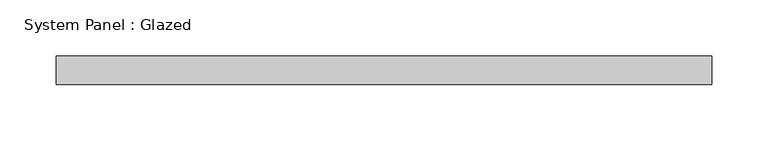
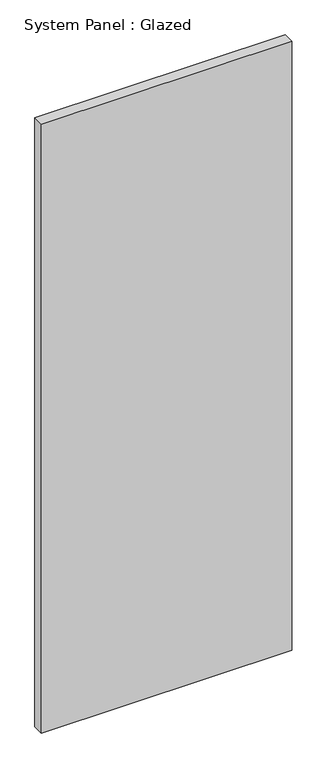
"""IFC4 building model written with IfcOpenShell, lengths in millimetres: plate geometry, System Panel : Glazed."""

from ifc_helpers import new_model, si_unit, origin, origin_with_axes, place, context, project, spatial, polyline, outline, extrude, source, transform, mapped, element, save


def system_panel_glazed_06fe117f(model_context):
    return source(origin(), model_context, "Body", "SweptSolid", [
        extrude(outline(polyline([(292.1, 19.05), (-292.1, 19.05), (-292.1, 44.45), (292.1, 44.45), (292.1, 19.05)])), origin_with_axes(), (0.0, 0.0, 1.0), 1502.0255085),
    ])


if __name__ == "__main__":
    model = new_model("IFC4")
    model_context = context("Model", 3, world=origin())
    ifc_project = project(units=[si_unit("LENGTHUNIT", "METRE", prefix="MILLI")], contexts=[model_context])
    site = spatial("IfcSite", under=ifc_project)
    building = spatial("IfcBuilding", under=site)
    placement = place(None, origin())
    system_panel_glazed_shape = system_panel_glazed_06fe117f(model_context)
    element("IfcPlate", 1, ObjectType="System Panel : Glazed", at=placement, inside=building, context=model_context, shape_type="MappedRepresentation", body=[
        mapped(system_panel_glazed_shape, transform((0.0, 0.0, 0.0), x_axis=(1.0, 0.0, 0.0), y_axis=(0.0, 1.0, 0.0), z_axis=(0.0, 0.0, 1.0))),
    ])
    save(model, "model.ifc")

# Revit data of these elements
# Type "System Panel : Glazed"
#   Construction Type Id = "GSP4R"
#   Analytic Construction = "1/8 in Pilkington single glazing"
#   Visual Light Transmittance = 0.9
#   Solar Heat Gain Coefficient = 0.86
#   Heat Transfer Coefficient (U) = 1.18115 BTU/(h·ft²·°F)
#   Define Thermal Properties by = 1
# Element 1 (IfcPlate, "System Panel : Glazed")
#   Materials on its faces: "Glass"
# Materials
#   "Glass": class "Glass", colour RGB 0 128 192, transparency 0.75, Description = "Soda Lime Glass", Cost = 0
